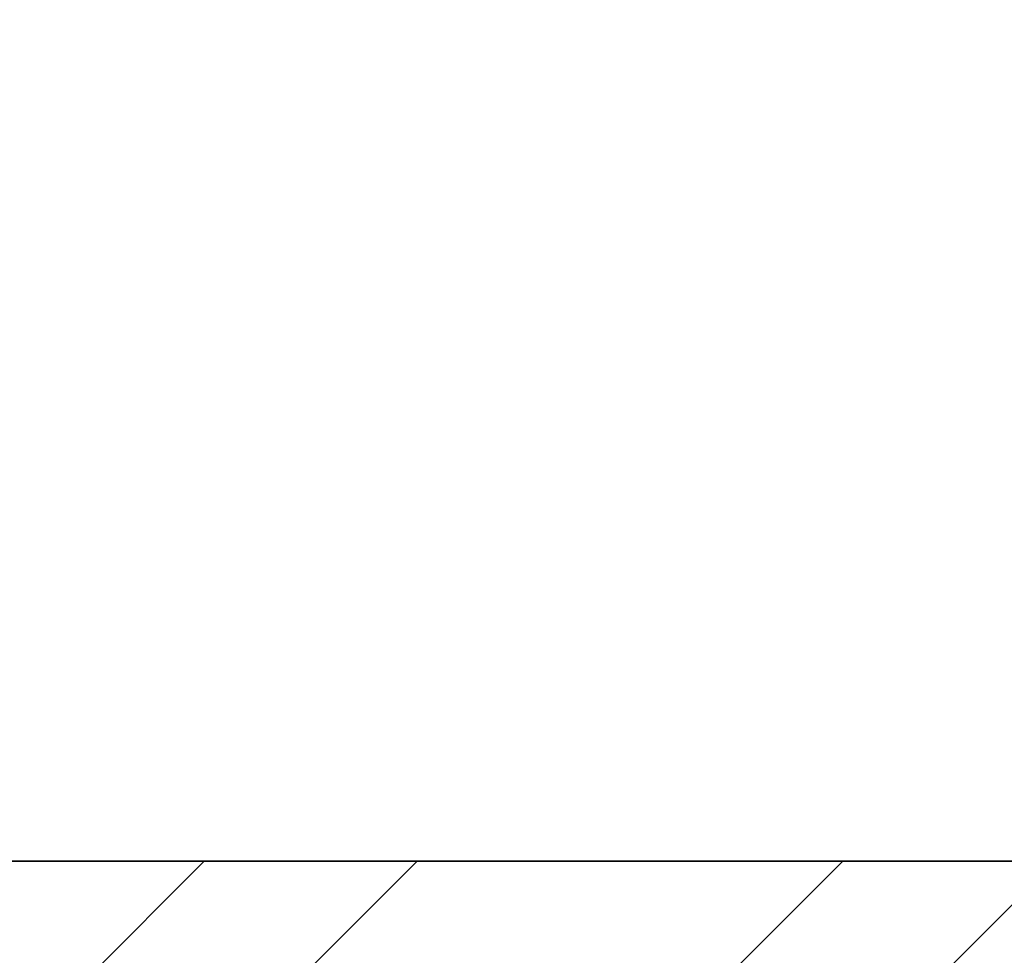
# Model space of a CAD drawing. Units: inches. Extents: x 1885 to 2748, y 783 to 2421.
# Tile 72 of 117: x 2017 to 2038, y 2073 to 2093. Entities that reach past the tile are written whole.
import ezdxf

# ---------------------------------------------------------------- set-up
doc = ezdxf.new("R2010")
doc.units = ezdxf.units.IN
doc.layers.add('A-WALL', color=7, linetype='Continuous', lineweight=35)
doc.layers.add('A-WALL-PATT', color=85, linetype='Continuous', lineweight=13, true_color=0x58ba48)

msp = doc.modelspace()

# ---------------------------------------------------------------- hatches: boundary and pattern name
at = {"layer": 'A-WALL-PATT'}
h = msp.add_hatch(dxfattribs=at)
h.set_pattern_fill('ANSI32', color=256)
h.paths.add_polyline_path([(2007.772, 2318.006), (1980.774, 2318.006), (1980.774, 2281.215), (1985.274, 2281.215), (1985.274, 2313.506), (2007.772, 2313.506), (2007.772, 2315.756)])
h.paths.add_polyline_path([(2094.324, 2318.006), (2067.772, 2318.006), (2067.772, 2313.506), (2094.324, 2313.506), (2094.324, 2315.756)])
h.paths.add_polyline_path([(2131.367, 2315.756), (2131.367, 2318.006), (2131.189, 2318.006), (2112.609, 2318.006), (2112.609, 2313.506), (2117.274, 2313.506), (2117.274, 2255.201), (2121.774, 2255.201), (2121.774, 2313.506), (2131.367, 2313.506)])
h.paths.add_polyline_path([(2190.512, 2318.006), (2155.367, 2318.006), (2155.367, 2313.506), (2169.774, 2313.506), (2169.774, 2229.506), (2121.774, 2229.506), (2121.774, 2233.451), (2119.524, 2233.451), (2117.274, 2233.451), (2117.274, 2201.101), (2121.774, 2201.101), (2121.774, 2225.006), (2169.774, 2225.006), (2169.774, 2165.006), (2306.274, 2165.006), (2306.274, 2066.006), (2310.774, 2066.006), (2344.274, 2066.006), (2486.274, 2066.006), (2486.274, 1886.006), (2483.02, 1886.006), (2483.02, 1881.506), (2486.274, 1881.506), (2486.274, 1880.678), (2490.774, 1880.678), (2490.774, 2070.506), (2344.274, 2070.506), (2310.774, 2070.506), (2310.774, 2165.006), (2310.774, 2173.636), (2308.524, 2173.636), (2306.274, 2173.636), (2306.274, 2169.506), (2174.274, 2169.506), (2174.274, 2313.506), (2190.512, 2313.506), (2190.512, 2315.756)])
h.paths.add_polyline_path([(1985.274, 2221.215), (1980.774, 2221.215), (1980.774, 2165.006), (1992.774, 2165.006), (1992.774, 2141.927), (1997.274, 2141.927), (1997.274, 2165.006), (2117.274, 2165.006), (2117.274, 2163.126), (2121.774, 2163.126), (2121.774, 2172.734), (2119.524, 2172.734), (2117.274, 2172.734), (2117.274, 2169.506), (1985.274, 2169.506)])
h.paths.add_polyline_path([(1997.274, 2105.927), (1992.774, 2105.927), (1992.774, 2070.506), (2016.774, 2070.506), (2016.774, 2059.123), (2019.024, 2059.123), (2021.274, 2059.123), (2021.274, 2070.506), (2117.274, 2070.506), (2117.274, 2022.506), (2114.423, 2022.506), (2114.423, 2018.006), (2123.627, 2018.006), (2123.627, 2020.256), (2123.627, 2022.506), (2121.774, 2022.506), (2121.774, 2142.587), (2119.524, 2142.587), (2117.274, 2142.587), (2117.274, 2075.006), (1997.274, 2075.006)])
h.paths.add_polyline_path([(2092.029, 2020.256), (2092.029, 2022.506), (2021.274, 2022.506), (2021.274, 2035.123), (2016.774, 2035.123), (2016.774, 2018.006), (2016.774, 1978.784), (2021.274, 1978.784), (2021.274, 2018.006), (2092.029, 2018.006)])
h.paths.add_polyline_path([(2260.938, 2022.506), (2153.105, 2022.506), (2153.105, 2020.256), (2153.105, 2018.006), (2155.274, 2018.006), (2155.274, 1886.006), (2107.629, 1886.006), (2107.629, 1881.506), (2182.911, 1881.506), (2182.911, 1883.756), (2182.911, 1886.006), (2159.774, 1886.006), (2159.774, 2018.006), (2260.938, 2018.006), (2260.938, 2020.256)])
h.paths.add_polyline_path([(2047.629, 1883.756), (2047.629, 1886.006), (2021.274, 1886.006), (2021.274, 1918.784), (2019.024, 1918.784), (2016.774, 1918.784), (2016.774, 1881.506), (2047.629, 1881.506)])
h.paths.add_polyline_path([(2306.361, 1883.756), (2306.361, 1886.006), (2296.274, 1886.006), (2296.274, 1982.006), (2316.535, 1982.006), (2316.535, 1984.256), (2316.535, 1986.506), (2296.274, 1986.506), (2296.274, 2022.506), (2289.276, 2022.506), (2289.276, 2018.006), (2291.774, 2018.006), (2291.774, 1886.006), (2242.911, 1886.006), (2242.911, 1881.506), (2306.361, 1881.506)], flags=17)
h.paths.add_polyline_path([(1985.274, 1843.006), (2021.6, 1843.006), (2021.534, 1845.441), (2021.477, 1847.506), (1980.774, 1847.506), (1980.774, 1809.446), (1985.274, 1809.446)])
h.paths.add_polyline_path([(2131.482, 1845.256), (2131.482, 1847.506), (2081.534, 1847.506), (2081.534, 1843.006), (2117.274, 1843.006), (2117.274, 1784.147), (2119.524, 1784.147), (2121.774, 1784.147), (2121.774, 1843.006), (2131.482, 1843.006)])
h.paths.add_polyline_path([(2203.886, 1847.506), (2155.482, 1847.506), (2155.482, 1843.006), (2169.774, 1843.006), (2169.774, 1759.006), (2121.774, 1759.006), (2121.774, 1761.457), (2117.274, 1761.457), (2117.274, 1730.429), (2121.774, 1730.429), (2121.774, 1754.506), (2177.421, 1754.506), (2177.421, 1756.756), (2177.421, 1759.006), (2174.274, 1759.006), (2174.274, 1843.006), (2203.886, 1843.006)])
h.paths.add_polyline_path([(2335.554, 1845.256), (2335.554, 1847.506), (2239.886, 1847.506), (2239.886, 1843.006), (2306.274, 1843.006), (2306.274, 1759.006), (2199.486, 1759.006), (2199.486, 1754.506), (2310.774, 1754.506), (2310.774, 1843.006), (2335.554, 1843.006)])
h.paths.add_polyline_path([(2348.774, 2022.506), (2344.274, 2022.506), (2344.274, 1986.506), (2341.681, 1986.506), (2341.681, 1982.006), (2344.274, 1982.006), (2344.274, 1886.006), (2330.361, 1886.006), (2330.361, 1881.506), (2361.627, 1881.506), (2361.627, 1883.756), (2361.627, 1886.006), (2348.774, 1886.006)], flags=17)
h.paths.add_polyline_path([(2283.251, 2315.756), (2283.251, 2318.006), (2238.512, 2318.006), (2238.512, 2313.506), (2283.251, 2313.506)], flags=17)
h.paths.add_polyline_path([(2363.274, 2348.006), (2388.677, 2348.006), (2388.677, 2350.256), (2388.677, 2352.506), (2358.774, 2352.506), (2358.774, 2348.006), (2358.774, 2318.006), (2344.481, 2318.006), (2344.481, 2313.506), (2358.774, 2313.506), (2358.774, 2229.506), (2310.774, 2229.506), (2310.774, 2231.952), (2306.274, 2231.952), (2306.274, 2205.611), (2310.774, 2205.611), (2310.774, 2225.006), (2358.774, 2225.006), (2358.774, 2211.506), (2452.329, 2211.506), (2452.329, 2213.756), (2452.329, 2216.006), (2363.274, 2216.006), (2363.274, 2318.006)])
h.paths.add_polyline_path([(2310.774, 2313.506), (2320.481, 2313.506), (2320.481, 2315.756), (2320.481, 2318.006), (2302.728, 2318.006), (2302.728, 2313.506), (2306.274, 2313.506), (2306.274, 2251.076), (2310.774, 2251.076)], flags=17)
h.paths.add_polyline_path([(2490.774, 2352.506), (2486.274, 2352.506), (2448.677, 2352.506), (2448.677, 2348.006), (2486.274, 2348.006), (2486.274, 2318.006), (2486.274, 2216.006), (2481.78, 2216.006), (2481.78, 2211.506), (2486.274, 2211.506), (2486.274, 2165.006), (2493.289, 2165.006), (2493.289, 2167.256), (2493.289, 2169.506), (2490.774, 2169.506), (2490.774, 2313.506), (2494.429, 2313.506), (2494.429, 2318.006), (2490.774, 2318.006)])
h.paths.add_polyline_path([(2534.653, 2318.006), (2515.691, 2318.006), (2515.691, 2313.506), (2534.653, 2313.506), (2534.653, 2315.756)])
h.paths.add_polyline_path([(2618.274, 2318.006), (2594.653, 2318.006), (2594.653, 2313.506), (2613.774, 2313.506), (2613.774, 2281.706), (2618.274, 2281.706)])
h.paths.add_polyline_path([(2618.274, 2221.706), (2613.774, 2221.706), (2613.774, 2169.506), (2554.019, 2169.506), (2554.019, 2165.006), (2613.774, 2165.006), (2613.774, 2152.878), (2618.274, 2152.878)])
h.paths.add_polyline_path([(2618.274, 2128.878), (2616.024, 2128.878), (2613.774, 2128.878), (2613.774, 2117.006), (2529.774, 2117.006), (2529.774, 2165.006), (2532.848, 2165.006), (2532.848, 2169.506), (2522.867, 2169.506), (2522.867, 2165.006), (2525.274, 2165.006), (2525.274, 2117.006), (2525.274, 2112.506), (2525.274, 2108.576), (2529.774, 2108.576), (2529.774, 2112.506), (2613.774, 2112.506), (2613.774, 2080.19), (2618.274, 2080.19)])
h.paths.add_polyline_path([(2618.274, 2044.19), (2616.024, 2044.19), (2613.774, 2044.19), (2613.774, 2015.506), (2529.774, 2015.506), (2529.774, 2088.582), (2527.524, 2088.582), (2525.274, 2088.582), (2525.274, 2011.006), (2613.774, 2011.006), (2613.774, 1956.755), (2618.274, 1956.755)])
h.paths.add_polyline_path([(2618.274, 1881.506), (2618.274, 1896.755), (2613.774, 1896.755), (2613.774, 1881.506), (2613.774, 1847.506), (2592.715, 1847.506), (2592.715, 1843.006), (2613.774, 1843.006), (2613.774, 1765.006), (2613.774, 1760.506), (2609.621, 1760.506), (2609.621, 1756.006), (2613.774, 1756.006), (2613.774, 1660.006), (2608.544, 1660.006), (2608.544, 1655.506), (2613.774, 1655.506), (2613.774, 1508.158), (2618.274, 1508.158)])
h.paths.add_polyline_path([(2565.774, 1843.006), (2568.997, 1843.006), (2568.997, 1847.506), (2490.774, 1847.506), (2490.774, 1849.7), (2488.524, 1849.7), (2486.274, 1849.7), (2486.274, 1847.506), (2477.274, 1847.506), (2477.274, 1838.506), (2477.274, 1821.493), (2486.274, 1821.493), (2486.274, 1838.506), (2561.274, 1838.506), (2561.274, 1765.006), (2486.274, 1765.006), (2486.274, 1786.157), (2477.274, 1786.157), (2477.274, 1765.006), (2477.274, 1756.006), (2486.274, 1756.006), (2565.774, 1756.006), (2585.621, 1756.006), (2585.621, 1758.256), (2585.621, 1760.506), (2565.774, 1760.506), (2565.774, 1765.006)])
h.paths.add_polyline_path([(2486.274, 1651.006), (2561.274, 1651.006), (2561.274, 1567.006), (2486.274, 1567.006), (2486.274, 1591.321), (2477.274, 1591.321), (2477.274, 1567.006), (2477.274, 1558.006), (2477.274, 1555.439), (2481.774, 1555.439), (2481.774, 1558.006), (2568.653, 1558.006), (2568.653, 1560.256), (2568.653, 1562.506), (2565.774, 1562.506), (2565.774, 1655.506), (2584.544, 1655.506), (2584.544, 1657.756), (2584.544, 1660.006), (2565.774, 1660.006), (2486.274, 1660.006), (2477.274, 1660.006), (2477.274, 1651.006), (2477.274, 1632.989), (2486.274, 1632.989)])
h.paths.add_polyline_path([(2449.967, 1883.756), (2449.967, 1886.006), (2421.627, 1886.006), (2421.627, 1881.506), (2449.967, 1881.506)], flags=17)
h.paths.add_polyline_path([(2447.274, 1847.506), (2395.554, 1847.506), (2395.554, 1843.006), (2442.774, 1843.006), (2442.774, 1809.27), (2447.274, 1809.27)])
h.paths.add_polyline_path([(1985.274, 1749.446), (1980.774, 1749.446), (1980.774, 1694.504), (1985.274, 1694.504), (1985.274, 1694.506), (1986.897, 1694.506), (1986.897, 1697.78), (1986.897, 1699.006), (1985.274, 1699.006)])
h.paths.add_polyline_path([(2152.774, 1699.006), (2121.774, 1699.006), (2121.774, 1703.668), (2119.524, 1703.668), (2117.274, 1703.668), (2117.274, 1699.006), (2009.219, 1699.006), (2009.219, 1694.506), (2148.274, 1694.506), (2148.274, 1692.631), (2152.774, 1692.631)])
h.paths.add_polyline_path([(2016.274, 1694.506), (2011.774, 1694.506), (2011.774, 1558.006), (2040.806, 1558.006), (2040.806, 1560.256), (2040.806, 1562.506), (2016.274, 1562.506)])
h.paths.add_polyline_path([(2152.774, 1663.017), (2150.524, 1663.017), (2148.274, 1663.017), (2148.274, 1562.506), (2100.806, 1562.506), (2100.806, 1558.006), (2165.119, 1558.006), (2165.119, 1560.256), (2165.119, 1562.506), (2152.774, 1562.506), (2152.774, 1610.506), (2224.774, 1610.506), (2224.774, 1607.99), (2229.274, 1607.99), (2229.274, 1615.006), (2152.774, 1615.006)])
h.paths.add_polyline_path([(2238.613, 1560.256), (2238.613, 1562.506), (2229.274, 1562.506), (2229.274, 1588.756), (2227.024, 1588.763), (2224.774, 1588.771), (2224.774, 1562.506), (2189.119, 1562.506), (2189.119, 1558.006), (2238.613, 1558.006)])
h.paths.add_polyline_path([(2336.024, 1560.256), (2336.024, 1562.506), (2310.774, 1562.506), (2310.774, 1656.347), (2308.524, 1656.347), (2306.274, 1656.347), (2306.274, 1562.506), (2286.613, 1562.506), (2286.613, 1558.006), (2336.024, 1558.006)])
h.paths.add_polyline_path([(2447.274, 1690.968), (2445.024, 1690.968), (2442.774, 1690.968), (2442.774, 1687.006), (2306.274, 1687.006), (2306.274, 1680.75), (2310.774, 1680.75), (2310.774, 1682.506), (2442.774, 1682.506), (2442.774, 1562.506), (2396.024, 1562.506), (2396.024, 1558.006), (2447.274, 1558.006)])
h.paths.add_polyline_path([(2447.274, 1749.27), (2445.024, 1749.27), (2442.774, 1749.27), (2442.774, 1717.232), (2447.274, 1717.232)])
h.paths.add_polyline_path([(2044.674, 1521.756), (2044.674, 1524.006), (2007.274, 1524.006), (2007.274, 1503.49), (2009.524, 1503.49), (2011.774, 1503.49), (2011.774, 1519.506), (2044.674, 1519.506)])
h.paths.add_polyline_path([(2177.969, 1521.756), (2177.969, 1524.006), (2104.674, 1524.006), (2104.674, 1519.506), (2145.774, 1519.506), (2145.774, 1387.506), (2143.37, 1387.506), (2143.37, 1383.006), (2251.585, 1383.006), (2251.585, 1385.256), (2251.585, 1387.506), (2150.274, 1387.506), (2150.274, 1519.506), (2177.969, 1519.506)])
h.paths.add_polyline_path([(2298.704, 1524.006), (2237.969, 1524.006), (2237.969, 1519.506), (2282.274, 1519.506), (2282.274, 1387.506), (2279.683, 1387.506), (2279.683, 1383.006), (2286.774, 1383.006), (2286.774, 1419.006), (2312.451, 1419.006), (2312.451, 1421.256), (2312.451, 1423.506), (2286.774, 1423.506), (2286.774, 1519.506), (2298.704, 1519.506), (2298.704, 1521.722)], flags=17)
h.paths.add_polyline_path([(2361.897, 1521.756), (2361.897, 1524.006), (2322.704, 1524.006), (2322.704, 1519.506), (2334.774, 1519.506), (2334.774, 1423.506), (2331.93, 1423.506), (2331.93, 1419.006), (2334.774, 1419.006), (2334.774, 1387.506), (2334.774, 1383.228), (2339.274, 1383.228), (2339.274, 1387.506), (2339.274, 1519.506), (2361.897, 1519.506)], flags=17)
h.paths.add_polyline_path([(2447.274, 1521.756), (2447.274, 1524.006), (2421.897, 1524.006), (2421.897, 1519.506), (2447.274, 1519.506)], flags=17)
h.paths.add_polyline_path([(2481.774, 1529.6), (2479.524, 1529.6), (2477.274, 1529.6), (2477.274, 1524.006), (2474.489, 1524.006), (2474.489, 1519.506), (2477.274, 1519.506), (2477.274, 1334.506), (2296.774, 1334.506), (2296.774, 1240.506), (2160.274, 1240.506), (2160.274, 1180.506), (2112.274, 1180.506), (2112.274, 1207.692), (2110.024, 1207.692), (2107.774, 1207.692), (2107.774, 1171.609), (2112.274, 1171.609), (2112.274, 1176.006), (2160.274, 1176.006), (2160.274, 1092.006), (2144.221, 1092.006), (2144.221, 1087.506), (2189.497, 1087.506), (2189.497, 1089.756), (2189.497, 1092.006), (2164.774, 1092.006), (2164.774, 1236.006), (2296.774, 1236.006), (2296.774, 1231.912), (2301.274, 1231.912), (2301.274, 1330.006), (2481.774, 1330.006), (2481.774, 1387.506)])
h.paths.add_polyline_path([(2618.274, 1448.158), (2613.774, 1448.158), (2613.774, 1382.506), (2529.774, 1382.506), (2525.274, 1382.506), (2525.274, 1307.062), (2529.774, 1307.062), (2529.774, 1378.006), (2613.774, 1378.006), (2613.774, 1354.988), (2618.274, 1354.988)])
h.paths.add_polyline_path([(2618.274, 1318.988), (2613.774, 1318.988), (2613.774, 1281.006), (2529.774, 1281.006), (2529.774, 1283.786), (2527.524, 1283.786), (2525.274, 1283.786), (2525.274, 1228.506), (2516.794, 1228.506), (2516.794, 1224.006), (2533.484, 1224.006), (2533.484, 1226.256), (2533.484, 1228.506), (2529.774, 1228.506), (2529.774, 1276.506), (2613.774, 1276.506), (2613.774, 1266.02), (2618.274, 1266.02)])
h.paths.add_polyline_path([(2618.274, 1134.964), (2613.774, 1134.964), (2613.774, 1092.006), (2594.545, 1092.006), (2594.545, 1087.506), (2618.274, 1087.506)])
h.paths.add_polyline_path([(2534.545, 1092.006), (2509.765, 1092.006), (2509.765, 1087.506), (2534.545, 1087.506), (2534.545, 1089.756)])
h.paths.add_polyline_path([(2481.274, 1224.006), (2484.117, 1224.006), (2484.117, 1226.256), (2484.117, 1228.506), (2476.774, 1228.506), (2476.774, 1198.506), (2471.61, 1198.506), (2471.61, 1194.006), (2476.774, 1194.006), (2476.774, 1062.006), (2436.894, 1062.006), (2436.894, 1057.506), (2476.774, 1057.506), (2481.274, 1057.506), (2481.274, 1062.006), (2481.274, 1087.506), (2485.354, 1087.506), (2485.354, 1089.756), (2485.354, 1092.006), (2481.274, 1092.006), (2481.274, 1117.506)])
h.paths.add_polyline_path([(2439.898, 1198.506), (2349.274, 1198.506), (2349.274, 1194.006), (2349.274, 1180.506), (2301.274, 1180.506), (2301.274, 1201.896), (2299.024, 1201.896), (2296.774, 1201.896), (2296.774, 1172.335), (2299.024, 1172.335), (2301.274, 1172.335), (2301.274, 1176.006), (2349.274, 1176.006), (2349.274, 1092.006), (2334.452, 1092.006), (2334.452, 1087.506), (2349.274, 1087.506), (2349.274, 1057.506), (2353.774, 1057.506), (2376.894, 1057.506), (2376.894, 1059.756), (2376.894, 1062.006), (2353.774, 1062.006), (2353.774, 1087.506), (2353.774, 1180.506), (2353.774, 1194.006), (2439.898, 1194.006), (2439.898, 1196.256)])
h.paths.add_polyline_path([(2270.596, 1089.756), (2270.596, 1092.006), (2249.497, 1092.006), (2249.497, 1087.506), (2270.596, 1087.506)], flags=17)
h.paths.add_polyline_path([(2310.452, 1092.006), (2301.274, 1092.006), (2301.274, 1153.292), (2296.774, 1153.292), (2296.774, 1092.006), (2293.786, 1092.006), (2293.786, 1087.506), (2310.452, 1087.506), (2310.452, 1089.756)], flags=17)
h.paths.add_polyline_path([(2112.274, 1150.328), (2110.024, 1150.328), (2107.774, 1150.328), (2107.774, 1092.006), (2104.465, 1092.006), (2104.465, 1087.506), (2120.221, 1087.506), (2120.221, 1089.756), (2120.221, 1092.006), (2112.274, 1092.006)])
h.paths.add_polyline_path([(2082.172, 1092.006), (2058.144, 1092.006), (2058.144, 1087.506), (2082.172, 1087.506), (2082.172, 1089.756)])
h.paths.add_polyline_path([(1975.774, 1145.638), (1971.274, 1145.638), (1971.274, 1087.506), (1980.774, 1087.506), (1998.144, 1087.506), (1998.144, 1089.756), (1998.144, 1092.006), (1985.274, 1092.006), (1975.774, 1092.006)])
h.paths.add_polyline_path([(2112.274, 1244.385), (2110.024, 1244.385), (2107.774, 1244.385), (2107.774, 1240.506), (1992.274, 1240.506), (1992.274, 1271.008), (1987.774, 1271.008), (1987.774, 1240.506), (1980.774, 1240.506), (1975.774, 1240.506), (1971.274, 1240.506), (1971.274, 1205.638), (1975.774, 1205.638), (1975.774, 1236.006), (2107.774, 1236.006), (2107.774, 1233.444), (2112.274, 1233.444), (2112.274, 1236.006)])
h.paths.add_polyline_path([(2112.274, 1383.006), (2114.783, 1383.006), (2114.783, 1385.256), (2114.783, 1387.506), (2102.476, 1387.506), (2102.476, 1383.006), (2107.774, 1383.006), (2107.774, 1335.006), (2011.774, 1335.006), (2011.774, 1349.939), (2007.274, 1349.939), (2007.274, 1335.006), (1987.774, 1335.006), (1987.774, 1330.506), (1987.774, 1307.008), (1992.274, 1307.008), (1992.274, 1330.506), (2007.274, 1330.506), (2107.774, 1330.506), (2107.774, 1264.711), (2112.274, 1264.711)])
h.paths.add_polyline_path([(2077.857, 1387.506), (2011.774, 1387.506), (2011.774, 1390.036), (2009.524, 1390.036), (2007.274, 1390.036), (2007.274, 1373.939), (2011.774, 1373.939), (2011.774, 1383.006), (2077.857, 1383.006)])
h.paths.add_polyline_path([(2011.774, 1443.49), (2007.274, 1443.49), (2007.274, 1410.248), (2011.774, 1410.248)])

# ---------------------------------------------------------------- linework, layer by layer
at = {"layer": 'A-WALL'}
msp.add_line((1997.274, 2075.006), (2117.274, 2075.006), dxfattribs=at)

doc.saveas('drawing.dxf')
